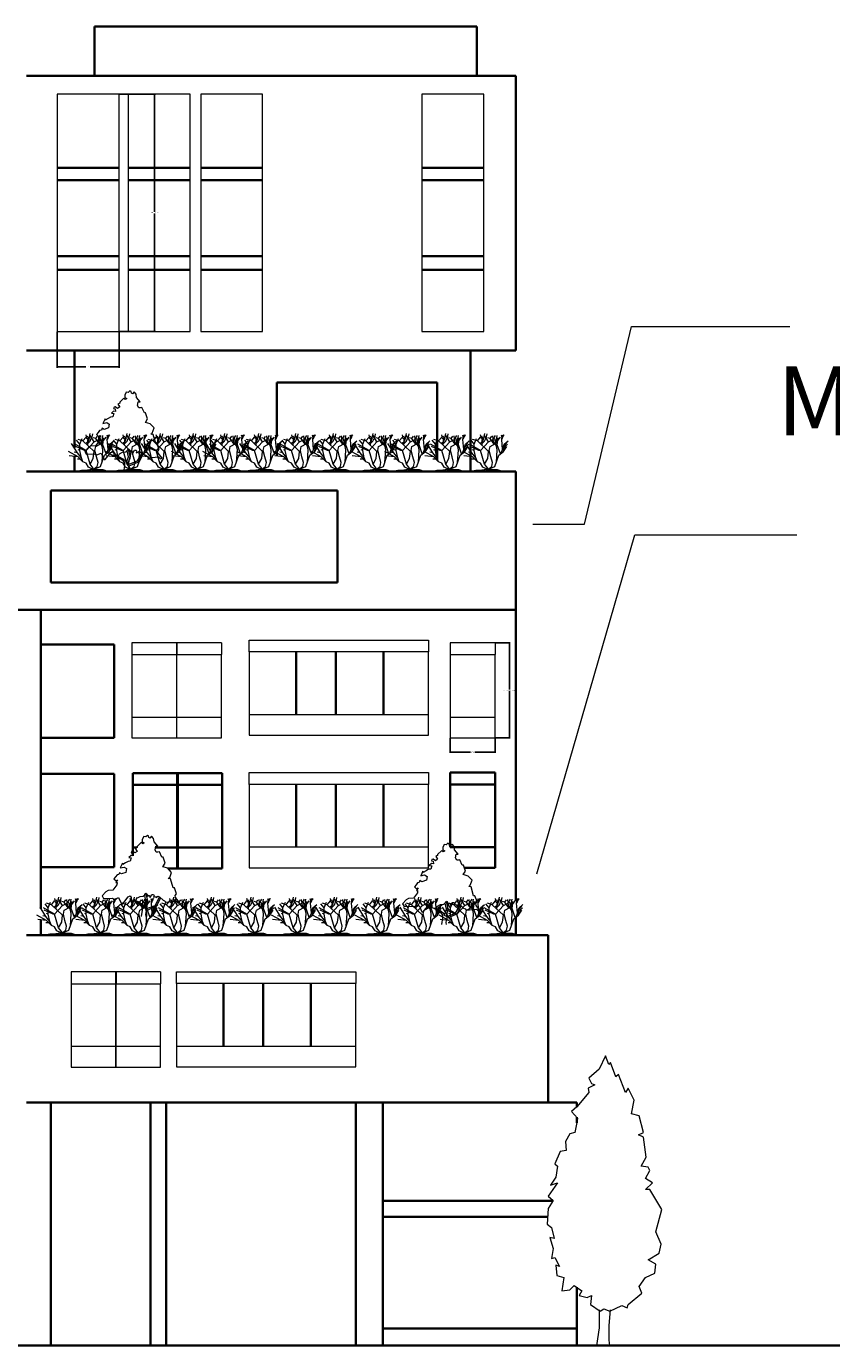
# Model space of a CAD drawing. Units: inches. Extents: x -1080 to 1950, y -1929 to 857.
# Tile 14 of 16: x 581 to 769, y 9 to 317. Entities that reach past the tile are written whole.
import ezdxf

# ---------------------------------------------------------------- set-up
doc = ezdxf.new("R2010")
doc.units = ezdxf.units.IN
doc.header["$MEASUREMENT"] = 0
for name, color, linetype, lineweight in [('A-ANNO-DIMS', 2, 'Continuous', 18), ('A-ANNO-SYMB', 2, 'Continuous', 18), ('A-ANNO-TEXT', 7, 'Continuous', 25), ('A-ELEV', 7, 'Continuous', 35), ('A-GLAZ', 4, 'Continuous', 18), ('L-PLNT', 82, 'Continuous', 13)]:
    doc.layers.add(name, color=color, linetype=linetype, lineweight=lineweight)
doc.styles.get("Standard").update_dxf_attribs({"font": 'arial.ttf'})
doc.dimstyles.get("Standard").update_dxf_attribs({"dimtxt": 0.18, "dimasz": 0.18, "dimexe": 0.18, "dimexo": 0.0625, "dimgap": 0.09, "dimtad": 0, "dimtih": 1, "dimtoh": 1, "dimdec": 4, "dimzin": 0, "dimdsep": 46, "dimtxsty": 'Standard', "dimcen": 0.09, "dimadec": 0, "dimazin": 0, "dimtfac": 1, "dimtdec": 4, "dimtofl": 0, "dimtmove": 0, "dimatfit": 3, "dimfxl": 1, "dimtolj": 1, "dimtzin": 0, "dimarcsym": 0})

# ---------------------------------------------------------------- blocks, each defined once
blk = doc.blocks.new('*U5')
blk.add_lwpolyline([(-2.754, 191.699), (-6.78, 182.851), (-13.682, 176.953), (-11.956, 173.266), (-9.656, 172.529), (-14.257, 170.317), (-13.682, 167.368), (-21.733, 157.783), (-25.184, 154.834), (-21.158, 150.41), (-21.733, 147.461), (-22.884, 140.825), (-26.334, 140.087), (-29.21, 134.926), (-28.635, 129.028), (-32.661, 128.291), (-36.111, 120.18), (-34.386, 118.706), (-35.536, 111.333), (-38.987, 106.171), (-34.386, 107.646), (-40.712, 98.798), (-37.261, 95.849), (-40.712, 90.688), (-41.287, 80.366), (-38.412, 78.154), (-36.686, 70.781), (-39.562, 71.518), (-37.261, 64.145), (-38.412, 57.509), (-36.111, 58.247), (-33.236, 52.348), (-35.536, 53.086), (-34.961, 46.45), (-30.36, 44.975), (-31.51, 36.128), (-26.334, 36.865), (-23.459, 39.814), (-18.283, 36.128), (-20.008, 33.178), (-14.832, 31.704), (-11.956, 33.178), (-12.531, 27.28), (-6.205, 22.856), (-3.905, 24.331), (0.121, 22.856), (8.173, 26.543), (11.624, 25.068), (12.199, 27.28), (21.4, 34.653), (19.675, 39.077), (23.701, 44.975), (30.027, 47.924), (30.602, 53.823), (25.426, 56.772), (32.903, 61.196), (34.053, 67.094), (30.602, 75.205), (34.628, 89.951), (26.576, 103.222), (23.701, 103.222), (28.302, 107.646), (23.701, 110.595), (26.576, 115.756), (25.426, 117.968), (20.825, 118.706), (24.276, 124.604), (22.551, 137.876), (19.1, 139.35), (22.551, 140.825), (19.675, 151.884), (14.499, 153.359), (16.224, 162.207), (12.199, 170.317), (10.473, 167.368), (5.872, 179.165), (4.147, 177.69), (0.696, 187.275), (-0.454, 185.8)], close=True)
for points in [[(-6.813, 23.669), (-6.813, 11.669), (-8.627, 0)], [(0.387, 23.669), (-0.576, 13.271), (-0.576, 3.686), (0, 0)]]:
    blk.add_lwpolyline(points)
blk = doc.blocks.new('*U6')
for p, q in [((-463.296, 280.416), (-552.577, 423.037)), ((-329.184, 316.992), (-499.872, 414.528)), ((-426.72, 414.528), (-475.488, 475.488)), ((-377.952, 463.296), (-451.104, 487.68)), ((-426.72, 414.528), (-390.144, 499.872)), ((-426.72, 316.992), (-426.72, 414.528)), ((-377.952, 463.296), (-329.184, 524.256)), ((-207.264, 304.8), (-377.952, 463.296)), ((-338.455, 424.7896), (-290.3982, 464.5406)), ((-329.184, 316.992), (-207.264, 451.104)), ((-316.7634, 502.285), (-327.6092, 559.9176)), ((-296.5958, 484.4034), (-316.7634, 502.285)), ((-286.512, 498.3226), (-307.4416, 538.0736)), ((-305.8922, 396.9512), (-302.7934, 478.4344)), ((-304.3428, 426.7708), (-268.7066, 458.5716)), ((-302.7934, 478.4344), (-270.256, 518.1854)), ((-290.3982, 464.5406), (-265.6078, 577.8246)), ((-268.7066, 458.5716), (-250.0884, 500.3038)), ((-207.264, 451.104), (-268.224, 548.64)), ((-240.792, 502.285), (-228.3968, 573.8368)), ((-182.88, 499.872), (-219.456, 512.064)), ((-207.264, 451.104), (-134.112, 487.68)), ((-182.88, 499.872), (-158.496, 536.448)), ((-121.92, 414.528), (-182.88, 499.872)), ((-182.88, 377.952), (-97.536, 426.72)), ((-129.1844, 450.6214), (-140.0302, 542.036)), ((-134.112, 487.68), (-97.536, 548.64)), ((-85.7758, 389.001), (-129.1844, 452.6026)), ((-73.152, 329.184), (-109.728, 499.872)), ((-97.536, 426.72), (-24.384, 524.256)), ((-85.7758, 472.4908), (-73.3552, 548.005)), ((-70.2564, 426.7708), (-85.7758, 472.4908)), ((-73.152, 402.336), (-60.96, 512.064)), ((-12.9032, 555.9552), (-2.0574, 522.1732)), ((-5.1562, 486.3846), (2.5908, 542.036)), ((8.7884, 335.3562), (-5.1562, 486.3846)), ((-3.6068, 492.3536), (14.986, 518.1854)), ((-0.508, 508.254), (22.7584, 536.067)), ((1.0414, 526.1356), (35.1536, 559.9176)), ((2.5908, 542.036), (21.209, 555.9552)), ((8.7884, 335.3562), (33.6042, 412.8516)), ((33.6042, 412.8516), (92.5068, 464.5406)), ((36.576, 390.144), (73.152, 438.912)), ((60.96, 390.144), (85.344, 414.528)), ((-451.104, 219.456), (-601.0402, 303.8094)), ((-451.104, 219.456), (-587.4512, 234.2388)), ((-463.296, 280.416), (-512.064, 292.608)), ((-353.568, 316.992), (-487.68, 377.952)), ((-402.336, 207.264), (-463.296, 280.416)), ((-426.72, 316.992), (-451.104, 329.184)), ((-377.952, 146.304), (-451.104, 219.456)), ((-402.336, 207.264), (-426.72, 316.992)), ((-377.952, 146.304), (-402.336, 207.264)), ((-329.184, 316.992), (-353.568, 316.992)), ((-268.224, 109.728), (-329.184, 316.992)), ((-219.456, 195.072), (-207.264, 304.8)), ((-195.072, 316.992), (-182.88, 377.952)), ((-170.688, 219.456), (-195.072, 316.992)), ((-146.304, 134.112), (-170.688, 219.456)), ((-109.728, 73.152), (-48.768, 243.84)), ((-85.344, 134.112), (-73.152, 329.184)), ((-24.384, 268.224), (-73.152, 402.336)), ((-48.768, 243.84), (24.384, 304.8)), ((-12.192, 274.32), (8.7884, 335.3562)), ((24.384, 304.8), (36.576, 390.144)), ((24.384, 304.8), (73.152, 377.952)), ((48.768, 341.376), (60.96, 390.144)), ((-414.528, 182.88), (-463.296, 182.88)), ((-402.336, 12.192), (-451.104, 0)), ((-341.376, 12.192), (-402.336, 12.192)), ((-329.184, 121.92), (-377.952, 146.304)), ((-243.84, 24.384), (-341.376, 12.192)), ((-292.608, 60.96), (-329.184, 121.92)), ((-243.84, 24.384), (-329.184, 0)), ((-219.456, 24.384), (-292.608, 60.96)), ((-268.224, 109.728), (-219.456, 195.072)), ((-219.456, 48.768), (-268.224, 109.728)), ((-243.84, 24.384), (-195.072, 24.384)), ((-219.456, 24.384), (-109.728, 73.152)), ((-219.456, 24.384), (-158.496, 73.152)), ((-219.456, 24.384), (-219.456, 48.768)), ((-219.456, 24.384), (-73.152, 24.384)), ((-195.072, 24.384), (-158.496, 12.192)), ((-158.496, 73.152), (-146.304, 134.112)), ((-158.496, 12.192), (-85.344, 0)), ((-73.152, 24.384), (0, 0))]:
    blk.add_line(p, q)
blk = doc.blocks.new('*U4')
for points in [[(559.11496, 3498.1134), (471.1065, 3595.68496), (394.41628, 3511.41284), (350.59112, 3539.5027), (339.63356, 3609.72862), (284.85592, 3637.82356), (208.16316, 3567.59256), (120.51538, 3581.63876), (54.78018, 3455.22804), (54.78018, 3342.86352), (142.42796, 3300.72746), (76.69022, 3258.58886), (10.95502, 3314.77366), (-175.2981, 3132.17814), (-175.2981, 3090.04208), (-251.98832, 3047.90602), (-230.07574, 3005.76742), (-175.2981, 2921.4953), (-273.9009, 2851.26684), (-372.50624, 2921.4953), (-427.28388, 2907.4491), (-449.19646, 2851.26684), (-372.50624, 2837.22064), (-361.54868, 2724.85612), (-447.2051, 2738.89978), (-547.79926, 2640.58146), (-438.24144, 2626.53526), (-482.06406, 2486.07834), (-580.66686, 2472.03214), (-690.22722, 2401.80622), (-821.70016, 2331.57776), (-832.65518, 2387.76002), (-931.26052, 2177.07464), (-755.96496, 2219.2107), (-646.4046, 2148.98224), (-679.2722, 1980.43546), (-876.4778, 1910.207), (-964.12812, 1966.38926), (-996.99572, 1882.1146), (-1073.68594, 1868.07094), (-1139.42368, 1783.79628), (-1216.11644, 1685.47796), (-1117.5111, 1601.2033), (-1051.7759, 1643.3419), (-1126.09884, 1521.20092), (-1072.10606, 1527.49758), (-1079.90386, 1416.93646), (-1259.93906, 1179.83508), (-1479.05978, 1165.78888), (-1577.66258, 1109.60662), (-1742.00312, 927.01364), (-1676.26538, 814.64658), (-1270.89408, 828.69278), (-1194.20386, 772.51052), (-1007.95074, 856.78518), (-876.4778, 575.87134), (-821.70016, 575.87134), (-569.71184, 884.87504), (-493.01908, 927.01364), (-438.24144, 856.78518), (-438.24144, 758.46432), (-350.59112, 730.37446), (-230.07574, 730.37446), (-186.25312, 828.69278), (-43.82516, 898.92124), (98.60534, 912.96744), (164.34054, 969.1497), (175.29556, 983.1959), (208.16316, 1053.42436), (251.98832, 1025.33196), (284.85592, 912.96744), (361.54614, 955.1035), (383.45872, 927.01364), (405.3713, 856.78518), (482.06406, 983.1959), (558.75428, 983.1959), (591.62188, 927.01364), (558.75428, 870.83138), (646.40206, 898.92124), (679.2722, 856.78518), (755.96242, 912.96744), (832.65518, 884.87504), (986.03816, 730.37446), (1051.77336, 702.28206), (1106.55354, 646.0998), (1566.70502, 688.23586), (1654.3528, 603.96374), (1720.09054, 632.0536), (1544.79244, 856.78518), (1533.83742, 941.0573), (1588.6176, 1025.33196), (1490.0148, 1292.1996), (1435.23462, 1292.1996), (1325.67426, 1685.47796), (1216.1139, 1699.52162), (1281.8491, 1755.70388), (1369.49688, 1980.43546), (1194.20132, 2163.02844), (975.08314, 2233.2569), (1073.68594, 2387.76002)], [(1073.68594, 2387.76002), (986.03816, 2654.62766), (931.25798, 2654.62766), (821.69762, 2893.4029), (755.96242, 2879.3567), (679.2722, 2879.3567), (624.48948, 2991.72376), (657.35708, 3146.22434), (745.0074, 3146.22434), (580.66686, 3342.86352), (558.75428, 3497.36664)], [(-328.67854, 730.37446), (-65.7352, 561.82514), (21.91004, 449.46062), (43.82262, 294.9575), (0, 0)], [(-251.98832, 716.32826), (0, 589.91754), (87.64778, 505.64288), (120.51538, 393.27836), (219.11818, 688.23586), (164.34054, 955.1035)], [(876.48034, 842.73898), (690.22722, 463.50682), (230.07574, 266.86764), (197.20814, 98.31832), (208.16316, 0)], [(208.16316, 1025.33196), (284.85592, 702.28206), (208.16316, 351.1423), (624.48948, 505.64288), (832.65518, 870.83138)]]:
    blk.add_lwpolyline(points)
blk = doc.blocks.new('WIN-TYPE-B')
for p, q in [((10.5, 22.21), (0, 22.21)), ((0, 22.21), (0, 19.45)), ((20.91, 22.21), (10.41, 22.21)), ((10.41, 22.21), (10.41, 19.45)), ((10.5, 22.21), (10.5, 19.45)), ((20.91, 22.21), (20.91, 19.45)), ((0, 19.45), (0, 4.84)), ((0, 19.45), (10.5, 19.45)), ((10.41, 19.45), (10.41, 4.84)), ((10.41, 19.45), (20.91, 19.45)), ((10.5, 4.84), (10.5, 19.45)), ((20.91, 4.84), (20.91, 19.45)), ((0, 4.84), (10.5, 4.84)), ((0, 4.84), (0, 0)), ((10.41, 4.84), (20.91, 4.84)), ((10.41, 4.84), (10.41, 0)), ((10.5, 0), (10.5, 4.84)), ((20.91, 0), (20.91, 4.84)), ((0, 0), (10.5, 0)), ((10.41, 0), (20.91, 0))]:
    blk.add_line(p, q)
blk = doc.blocks.new('WIN-TYPE-E')
for p, q in [((10.5, 22.21), (0, 22.21)), ((0, 22.21), (0, 19.45)), ((10.5, 22.21), (10.5, 19.45)), ((0, 19.45), (0, 4.84)), ((0, 19.45), (10.5, 19.45)), ((10.5, 4.84), (10.5, 19.45)), ((0, 4.84), (10.5, 4.84)), ((0, 4.84), (0, 0)), ((10.5, 0), (10.5, 4.84)), ((0, 0), (10.5, 0))]:
    blk.add_line(p, q)
blk = doc.blocks.new('WIN-TYPE-G')
for p, q in [((0, 19.45), (0, 22.21)), ((0, 22.21), (41.85, 22.21)), ((41.85, 22.21), (41.85, 19.45)), ((0, 19.45), (0, 4.84)), ((41.85, 19.45), (0, 19.45)), ((41.85, 4.84), (41.85, 19.45)), ((0, 4.84), (41.85, 4.84)), ((0, 4.84), (0, 0)), ((41.85, 0), (41.85, 4.84)), ((0, 0), (41.85, 0))]:
    blk.add_line(p, q)
blk = doc.blocks.new('PANEL-B')
for p, q in [((0, 55.38), (0, 0)), ((14.46, 55.38), (0, 55.38)), ((14.46, 0), (14.46, 55.38)), ((0, 0), (14.46, 0))]:
    blk.add_line(p, q)
blk = doc.blocks.new('*D43')
at = {"layer": 'A-ANNO-DIMS', "color": 0, "lineweight": -2, "transparency": 16777216}
for p, q in [((690.47, 173), (693.92, 173)), ((693.74, 172.82), (693.74, 162.08)), ((693.74, 150.98), (693.74, 161.72)), ((690.47, 150.8), (693.92, 150.8))]:
    blk.add_line(p, q, dxfattribs=at)
at = {"layer": 'A-ANNO-DIMS', "color": 0, "transparency": 16777216}
for points in [[(693.71, 172.82), (693.77, 172.82), (693.74, 173)], [(693.71, 150.98), (693.77, 150.98), (693.74, 150.8)]]:
    blk.add_solid(points, dxfattribs=at)
at = {"layer": 'Defpoints', "color": 0, "transparency": 16777216}
for p in [(690.41, 173), (693.74, 173), (690.41, 150.8)]:
    blk.add_point(p, dxfattribs=at)
at = {"layer": 'A-ANNO-DIMS', "color": 0, "transparency": 16777216, "insert": (693.74, 161.9), "char_height": 0.18, "attachment_point": 5}
blk.add_mtext('\\A1;WINDOW TYPE E 22 TYP.', dxfattribs=at)
blk = doc.blocks.new('*D44')
at = {"layer": 'A-ANNO-DIMS', "color": 0, "lineweight": -2, "transparency": 16777216}
for p, q in [((679.91, 150.73), (679.91, 147.28)), ((690.41, 150.73), (690.41, 147.28)), ((680.09, 147.46), (684.64, 147.46)), ((690.23, 147.46), (685.68, 147.46))]:
    blk.add_line(p, q, dxfattribs=at)
at = {"layer": 'A-ANNO-DIMS', "color": 0, "transparency": 16777216}
for points in [[(680.09, 147.49), (680.09, 147.43), (679.91, 147.46)], [(690.23, 147.49), (690.23, 147.43), (690.41, 147.46)]]:
    blk.add_solid(points, dxfattribs=at)
at = {"layer": 'Defpoints', "color": 0, "transparency": 16777216}
for p in [(679.91, 150.8), (690.41, 150.8), (690.41, 147.46)]:
    blk.add_point(p, dxfattribs=at)
at = {"layer": 'A-ANNO-DIMS', "color": 0, "transparency": 16777216, "insert": (685.16, 147.46), "char_height": 0.18, "attachment_point": 5}
blk.add_mtext('\\A1;11 TYP.', dxfattribs=at)
blk = doc.blocks.new('*D73')
at = {"layer": 'A-ANNO-DIMS', "color": 0, "lineweight": -2, "transparency": 16777216}
for p, q in [((602.67, 301.01), (611.09, 301.01)), ((610.91, 300.83), (610.91, 273.51)), ((610.91, 245.81), (610.91, 273.14)), ((602.67, 245.63), (611.09, 245.63))]:
    blk.add_line(p, q, dxfattribs=at)
at = {"layer": 'A-ANNO-DIMS', "color": 0, "transparency": 16777216}
for points in [[(610.88, 300.83), (610.94, 300.83), (610.91, 301.01)], [(610.88, 245.81), (610.94, 245.81), (610.91, 245.63)]]:
    blk.add_solid(points, dxfattribs=at)
at = {"layer": 'Defpoints', "color": 0, "transparency": 16777216}
for p in [(602.61, 301.01), (610.91, 301.01), (602.61, 245.63)]:
    blk.add_point(p, dxfattribs=at)
at = {"layer": 'A-ANNO-DIMS', "color": 0, "transparency": 16777216, "insert": (610.91, 273.32), "char_height": 0.18, "attachment_point": 5}
blk.add_mtext('\\A1;PANEL B 55 TYP.', dxfattribs=at)
blk = doc.blocks.new('*D74')
at = {"layer": 'A-ANNO-DIMS', "color": 0, "lineweight": -2, "transparency": 16777216}
for p, q in [((588.15, 245.57), (588.15, 237.15)), ((602.61, 245.57), (602.61, 237.15)), ((588.33, 237.33), (594.86, 237.33)), ((602.43, 237.33), (595.9, 237.33))]:
    blk.add_line(p, q, dxfattribs=at)
at = {"layer": 'A-ANNO-DIMS', "color": 0, "transparency": 16777216}
for points in [[(588.33, 237.36), (588.33, 237.3), (588.15, 237.33)], [(602.43, 237.36), (602.43, 237.3), (602.61, 237.33)]]:
    blk.add_solid(points, dxfattribs=at)
at = {"layer": 'Defpoints', "color": 0, "transparency": 16777216}
for p in [(588.15, 245.63), (602.61, 245.63), (602.61, 237.33)]:
    blk.add_point(p, dxfattribs=at)
at = {"layer": 'A-ANNO-DIMS', "color": 0, "transparency": 16777216, "insert": (595.38, 237.33), "char_height": 0.18, "attachment_point": 5}
blk.add_mtext('\\A1;14 TYP.', dxfattribs=at)

msp = doc.modelspace()

# ---------------------------------------------------------------- linework, layer by layer
at = {"layer": 'A-ANNO-SYMB'}
for p, q in [((711.25, 200.63), (722.26, 246.75)), ((722.26, 246.75), (759.2, 246.75)), ((699.18, 200.63), (711.25, 200.63)), ((700.16, 119.09), (723.01, 198.18)), ((723.01, 198.18), (760.82, 198.18))]:
    msp.add_line(p, q, dxfattribs=at)
at = {"layer": 'A-ELEV'}
for p, q in [((596.9, 305.29), (596.9, 316.8)), ((596.9, 316.8), (686.12, 316.8)), ((686.12, 316.8), (686.12, 305.29)), ((580.98, 305.29), (695.2, 305.29)), ((695.2, 282.99), (695.2, 305.29)), ((588.15, 283.83), (602.61, 283.83)), ((604.78, 283.83), (619.24, 283.83)), ((621.67, 283.83), (636.13, 283.83)), ((673.31, 283.83), (687.76, 283.83)), ((588.15, 280.95), (602.61, 280.95)), ((604.78, 280.95), (619.24, 280.95)), ((621.67, 280.95), (636.13, 280.95)), ((673.31, 280.95), (687.76, 280.95)), ((695.2, 282.99), (695.2, 241.18)), ((588.15, 263.22), (602.61, 263.22)), ((604.78, 263.22), (619.24, 263.22)), ((621.67, 263.22), (636.13, 263.22)), ((673.31, 263.22), (687.76, 263.22)), ((588.15, 260.02), (602.61, 260.02)), ((604.78, 260.02), (619.24, 260.02)), ((621.67, 260.02), (636.13, 260.02)), ((673.31, 260.02), (687.76, 260.02)), ((592.18, 241.18), (580.98, 241.18)), ((580.98, 241.18), (695.2, 241.18)), ((592.18, 218.44), (592.18, 241.18)), ((684.65, 212.94), (684.65, 241.18)), ((639.41, 221.35), (639.41, 233.75)), ((639.41, 233.75), (676.84, 233.75)), ((676.84, 233.75), (676.84, 215.59)), ((592.18, 212.94), (592.18, 216.45)), ((639.41, 216.53), (639.41, 217.47)), ((580.98, 212.94), (695.2, 212.94)), ((676.84, 213.2), (676.84, 212.94)), ((695.2, 180.63), (695.2, 212.94)), ((695.2, 212.94), (695.2, 211.45)), ((695.2, 212.94), (695.2, 112.8)), ((653.62, 208.55), (586.68, 208.55)), ((586.68, 208.55), (586.68, 187.05)), ((653.62, 187.05), (653.62, 208.55)), ((586.68, 187.05), (653.62, 187.05)), ((478.29, 180.63), (695.2, 180.63)), ((584.39, 142.43), (584.39, 180.63)), ((584.39, 172.58), (601.46, 172.58)), ((584.39, 150.8), (584.39, 172.58)), ((601.46, 172.58), (601.46, 150.8)), ((643.95, 170.85), (643.95, 156.23)), ((653.22, 170.85), (653.22, 156.23)), ((664.33, 170.85), (664.33, 156.23)), ((601.46, 150.8), (584.39, 150.8)), ((584.39, 142.43), (601.46, 142.43)), ((584.39, 120.65), (584.39, 142.43)), ((601.46, 142.43), (601.46, 120.65)), ((616.31, 142.55), (605.8, 142.55)), ((605.8, 142.55), (605.8, 139.8)), ((626.71, 142.55), (616.21, 142.55)), ((616.21, 142.55), (616.21, 139.8)), ((616.31, 142.55), (616.31, 139.8)), ((626.71, 142.55), (626.71, 139.8)), ((690.41, 142.7), (679.91, 142.7)), ((679.91, 142.7), (679.91, 139.94)), ((690.41, 142.7), (690.41, 139.94)), ((605.8, 139.8), (605.8, 125.18)), ((605.8, 139.8), (616.31, 139.8)), ((616.21, 139.8), (616.21, 125.18)), ((616.21, 139.8), (626.71, 139.8)), ((616.31, 125.18), (616.31, 139.8)), ((626.71, 125.18), (626.71, 139.8)), ((643.95, 139.94), (643.95, 125.32)), ((653.22, 139.94), (653.22, 125.32)), ((664.33, 139.94), (664.33, 125.32)), ((679.91, 139.94), (679.91, 125.32)), ((679.91, 139.94), (690.41, 139.94)), ((690.41, 125.32), (690.41, 139.94)), ((605.8, 125.18), (606.8, 125.18)), ((605.8, 125.18), (605.8, 123.3)), ((611.11, 125.18), (616.31, 125.18)), ((616.21, 125.18), (626.71, 125.18)), ((616.21, 125.18), (616.21, 120.34)), ((616.31, 120.34), (616.31, 125.18)), ((626.71, 120.34), (626.71, 125.18)), ((679.91, 125.32), (690.41, 125.32)), ((690.41, 120.49), (690.41, 125.32)), ((601.46, 120.65), (584.39, 120.65)), ((584.39, 120.65), (584.39, 110.89)), ((613.99, 120.34), (616.31, 120.34)), ((616.21, 120.34), (626.71, 120.34)), ((683.22, 120.49), (690.41, 120.49)), ((695.45, 112.8), (695.69, 112.8)), ((584.39, 108.3), (584.39, 104.79)), ((695.2, 104.79), (695.2, 108.91)), ((580.98, 104.79), (695.2, 104.79)), ((695.2, 104.78), (702.79, 104.78)), ((702.79, 104.78), (702.79, 65.68)), ((627, 93.45), (627, 78.83)), ((636.26, 93.45), (636.26, 78.83)), ((647.38, 93.45), (647.38, 78.83)), ((702.79, 65.68), (580.98, 65.68)), ((586.66, 65.68), (586.66, 9.02)), ((609.98, 65.68), (609.98, 9.02)), ((613.6, 65.68), (613.6, 9.02)), ((657.88, 65.68), (657.88, 9.02)), ((664.2, 9.02), (664.2, 65.68)), ((709.45, 65.68), (699.18, 65.68)), ((702.79, 65.68), (702.79, 65.68)), ((702.79, 65.68), (702.79, 65.68)), ((702.79, 65.68), (702.79, 65.68)), ((709.45, 65.68), (709.45, 64.65)), ((709.45, 62.29), (709.45, 60.97)), ((664.2, 42.8), (703.97, 42.8)), ((664.2, 39), (702.65, 39)), ((709.45, 22.6), (709.45, 9.02)), ((664.2, 13.01), (709.45, 13.01)), ((709.45, 9.02), (-148.56, 9.02)), ((709.45, 9.02), (833.43, 9.02))]:
    msp.add_line(p, q, dxfattribs=at)

# ---------------------------------------------------------------- block references
at = {"layer": 'A-GLAZ'}
for name, p in [('PANEL-B', (588.15, 245.63)), ('PANEL-B', (604.78, 245.63)), ('PANEL-B', (621.67, 245.63)), ('PANEL-B', (673.31, 245.63)), ('WIN-TYPE-B', (605.61, 150.79)), ('WIN-TYPE-G', (632.99, 151.4)), ('WIN-TYPE-E', (679.91, 150.79)), ('WIN-TYPE-G', (632.99, 120.49)), ('WIN-TYPE-B', (591.41, 73.98)), ('WIN-TYPE-G', (616.03, 74))]:
    msp.add_blockref(name, p, dxfattribs=at)
at = {"layer": 'L-PLNT'}
for name, p, xscale, yscale, zscale in [('*U4', (603.68, 212.77), 0.0052143573184964, 0.0052143573184964, 0.0052143573184964), ('*U6', (599.95, 213.01), 0.0152219259934872, 0.0152219259934872, 0.0152219259934872), ('*U6', (608.57, 213.01), 0.0152219259934872, 0.0152219259934872, 0.0152219259934872), ('*U6', (616.3, 213.01), 0.0152219259934872, 0.0152219259934872, 0.0152219259934872), ('*U6', (624.02, 213.01), 0.0152219259934872, 0.0152219259934872, 0.0152219259934872), ('*U6', (631.35, 213.01), 0.0152219259934872, 0.0152219259934872, 0.0152219259934872), ('*U6', (639.25, 213.01), 0.0152219259934872, 0.0152219259934872, 0.0152219259934872), ('*U6', (647.91, 213.01), 0.0152219259934872, 0.0152219259934872, 0.0152219259934872), ('*U6', (656.69, 213.01), 0.0152219259934872, 0.0152219259934872, 0.0152219259934872), ('*U6', (665.98, 213.01), 0.0152219259934872, 0.0152219259934872, 0.0152219259934872), ('*U6', (673.78, 213.01), 0.0152219259934872, 0.0152219259934872, 0.0152219259934872), ('*U6', (682.95, 213.01), 0.0152219259934872, 0.0152219259934872, 0.0152219259934872), ('*U6', (692.01, 213.01), 0.0152219259934872, 0.0152219259934872, 0.0152219259934872), ('*U4', (607.75, 109.08), 0.0052143573184964, 0.0052143573184964, 0.0052143573184964), ('*U4', (677.89, 107.23), 0.0052143573184964, 0.0052143573184964, 0.0052143573184964), ('*U6', (592.58, 104.82), 0.0152219259934872, 0.0152219259934872, 0.0152219259934872), ('*U6', (601.47, 104.82), 0.0152219259934872, 0.0152219259934872, 0.0152219259934872), ('*U6', (610.23, 104.82), 0.0152219259934872, 0.0152219259934872, 0.0152219259934872), ('*U6', (619.45, 104.82), 0.0152219259934872, 0.0152219259934872, 0.0152219259934872), ('*U6', (628.24, 104.82), 0.0152219259934872, 0.0152219259934872, 0.0152219259934872), ('*U6', (637.46, 104.82), 0.0152219259934872, 0.0152219259934872, 0.0152219259934872), ('*U6', (647.37, 104.82), 0.0152219259934872, 0.0152219259934872, 0.0152219259934872), ('*U6', (656.96, 104.82), 0.0152219259934872, 0.0152219259934872, 0.0152219259934872), ('*U6', (666.82, 104.82), 0.0152219259934872, 0.0152219259934872, 0.0152219259934872), ('*U6', (676.61, 104.82), 0.0152219259934872, 0.0152219259934872, 0.0152219259934872), ('*U6', (686.5, 104.82), 0.0152219259934872, 0.0152219259934872, 0.0152219259934872), ('*U6', (695.49, 104.82), 0.0152219259934872, 0.0152219259934872, 0.0152219259934872), ('*U5', (717.12, 8.99), 0.3528399638811642, 0.3528399638811642, 0.3528399638811642)]:
    msp.add_blockref(name, p, dxfattribs=dict(at, xscale=xscale, yscale=yscale, zscale=zscale))

# ---------------------------------------------------------------- texts
at = {"layer": 'A-ANNO-TEXT'}
msp.add_text('MEETING   SPACE', height=16.1087, dxfattribs=at).set_placement((756.13, 221.37))

# ---------------------------------------------------------------- dimensions: what is measured, and where the dimension line sits
at = {"layer": 'A-ANNO-DIMS'}
for base, p1, p2, text, picture, middle in [((610.91, 301.01), (602.61, 245.63), (602.61, 301.01), 'PANEL B <> TYP.', '*D73', (610.91, 273.32)), ((693.74, 173), (690.41, 150.8), (690.41, 173), 'WINDOW TYPE E <> TYP.', '*D43', (693.74, 161.9))]:
    dim = msp.add_linear_dim(base=base, p1=p1, p2=p2, angle=90, text=text, dimstyle='Standard', override={"dimdec": 0, "dimlfac": 1, "dimrnd": 0, "dimzin": 0, "dimdsep": 46, "dimlunit": 2}, dxfattribs=at)
    dim.commit()
    dim.dimension.update_dxf_attribs({"geometry": picture, "text_midpoint": middle})
for base, p1, p2, picture, middle in [((602.61, 237.33), (588.15, 245.63), (602.61, 245.63), '*D74', (595.38, 237.33)), ((690.4085, 147.464), (679.906, 150.7953), (690.4085, 150.7953), '*D44', (685.1573, 147.464))]:
    dim = msp.add_linear_dim(base=base, p1=p1, p2=p2, text='<> TYP.', dimstyle='Standard', override={"dimdec": 0, "dimlfac": 1, "dimrnd": 0, "dimzin": 0, "dimdsep": 46, "dimlunit": 2}, dxfattribs=at)
    dim.commit()
    dim.dimension.update_dxf_attribs({"geometry": picture, "text_midpoint": middle})

doc.saveas('drawing.dxf')
